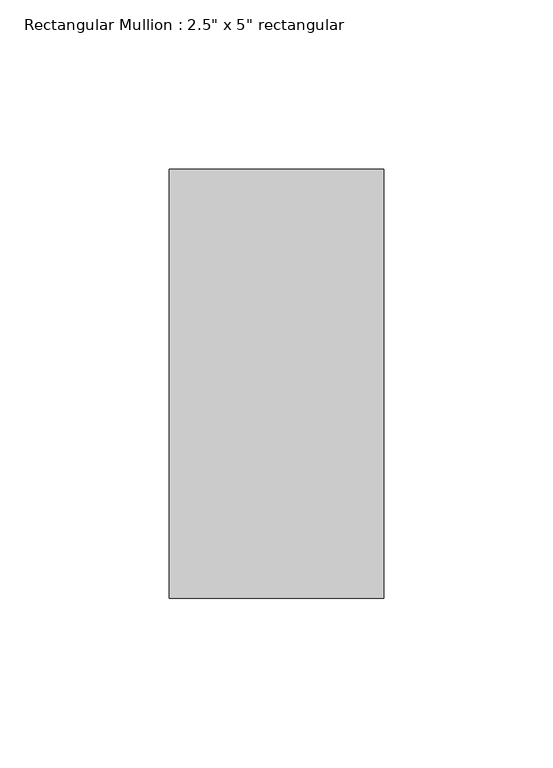
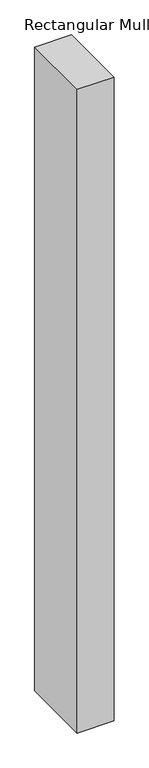
"""IFC4 building model written with IfcOpenShell, lengths in millimetres: member geometry."""

from ifc_helpers import new_model, si_unit, frame, origin, place, context, project, spatial, polyline, outline, extrude, source, transform, mapped, element, save


def member_5d96a33e(model_context):
    return source(origin(), model_context, "Body", "SweptSolid", [
        extrude(outline(polyline([(0.0, 63.5), (0.0, -63.5), (-63.5, -63.5), (-63.5, 63.5), (0.0, 63.5)])), frame((0.0, 0.0, -1174.7500001), z_axis=(0.0, 0.0, 1.0), x_axis=(1.0, 0.0, 0.0)), (0.0, 0.0, 1.0), 1174.7500001),
    ])


if __name__ == "__main__":
    model = new_model("IFC4")
    model_context = context("Model", 3, world=origin())
    ifc_project = project(units=[si_unit("LENGTHUNIT", "METRE", prefix="MILLI")], contexts=[model_context])
    site = spatial("IfcSite", under=ifc_project)
    building = spatial("IfcBuilding", under=site)
    placement = place(None, origin())
    member_shape = member_5d96a33e(model_context)
    element("IfcMember", 1, ObjectType="Rectangular Mullion : 2.5\" x 5\" rectangular", at=placement, inside=building, context=model_context, shape_type="MappedRepresentation", body=[
        mapped(member_shape, transform((0.0, 0.0, 0.0), x_axis=(1.0, 0.0, 0.0), y_axis=(0.0, 1.0, 0.0), z_axis=(0.0, 0.0, 1.0))),
    ])
    save(model, "model.ifc")

# Revit data of these elements
# Type "Rectangular Mullion : 2.5\" x 5\" rectangular"
#   built-in parameter 1007304 = 0.416667 (stored number, unit not read)
#   built-in parameter 1007301 = 0.104167 (stored number, unit not read)
#   built-in parameter 1007300 = 0.104167 (stored number, unit not read)
# Element 1 (IfcMember, "Rectangular Mullion : 2.5\" x 5\" rectangular")
#   Materials on its faces: "WINDOW FRAMING"
# Materials
#   "WINDOW FRAMING": class "Generic", colour RGB 120 120 120, transparency 0, Cost = 0
